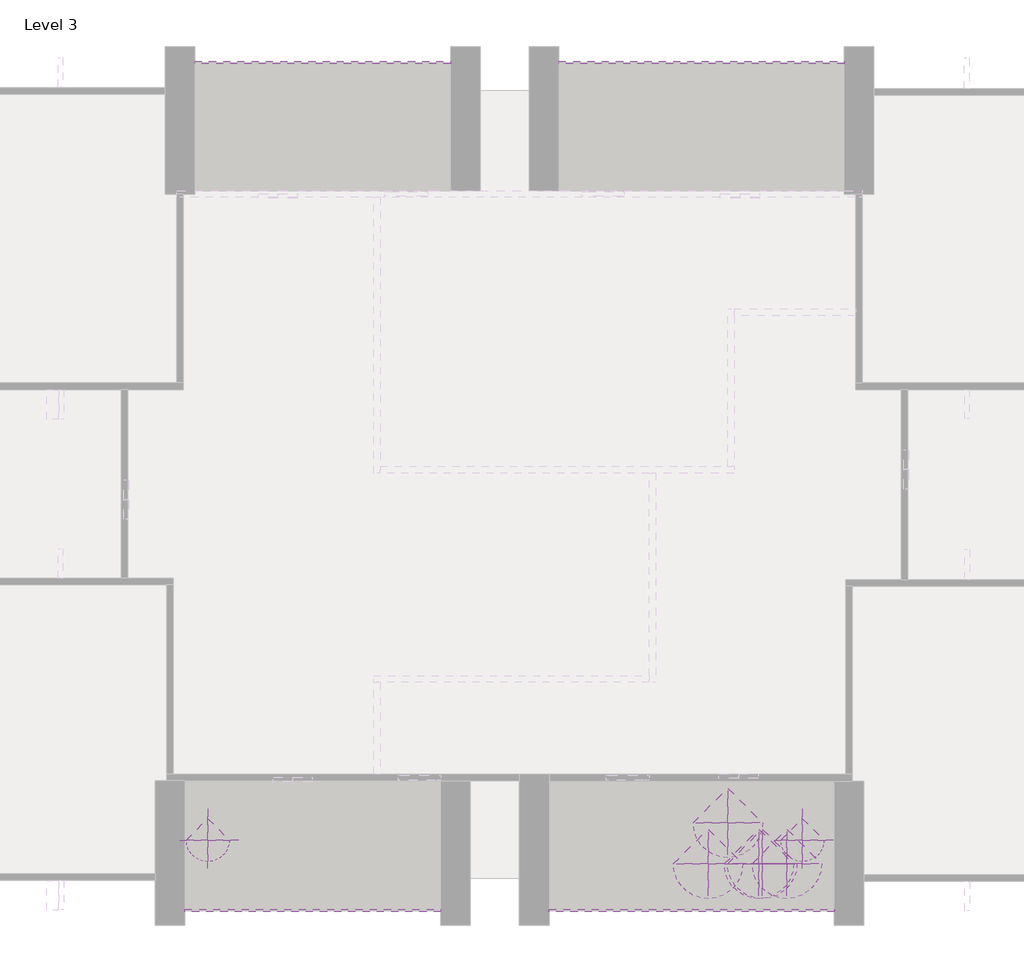
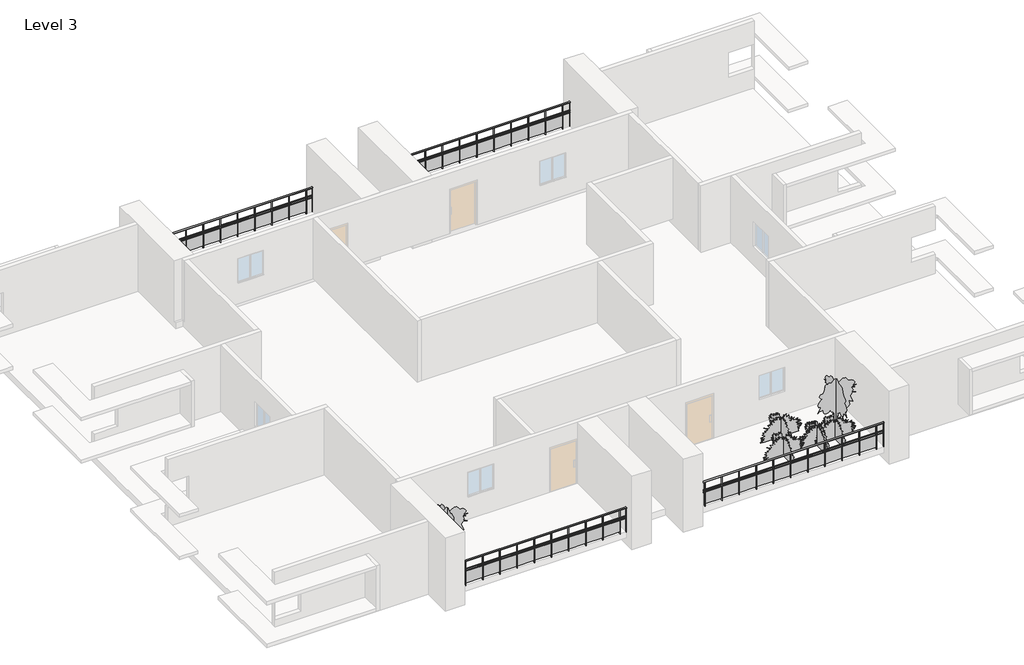
# One storey, part 4 of 4: 7 geographic elements, 4 railings.
"""IFC4 building model written with IfcOpenShell, lengths in millimetres."""

from ifc_helpers import new_model, si_unit, point, frame, origin, place, context, project, spatial, polyline, ellipse_curve, trimmed, outline, extrude, transform, mapped, element, save
from ifc_brep_helpers import plane_surface, extruded_surface, advanced_brep
from components import geographic_element_3d6ded1d, rpc_tree_tropical_d7a905c7

model = new_model("IFC4")

# Units and contexts
model_context = context("Model", 3, world=origin())
ifc_project = project(units=[si_unit("LENGTHUNIT", "METRE", prefix="MILLI")], contexts=[model_context])

# Site, building, storey
site = spatial("IfcSite", under=ifc_project)
building = spatial("IfcBuilding", under=site)
storey = spatial("IfcBuildingStorey", under=building, Name="Level 3", Elevation=6096.0)

# Geographic elements
placement = place(None, origin())
geographic_element_shape = geographic_element_3d6ded1d(model_context)
element("IfcGeographicElement", 1, ObjectType="RPC Shrub : Fountain Grass 3'-6\"", at=placement, inside=storey, context=model_context, shape_type="MappedRepresentation", body=[
    mapped(geographic_element_shape, transform((9500.2520665, -7929.230811, 7315.2), x_axis=(1.0, 0.0, 0.0), y_axis=(0.0, 1.0, 0.0), z_axis=(0.0, 0.0, 1.0))),
])
element("IfcGeographicElement", 2, ObjectType="RPC Shrub : Fountain Grass 3'-6\"", at=placement, inside=storey, context=model_context, shape_type="MappedRepresentation", body=[
    mapped(geographic_element_shape, transform((11938.6520665, -7929.230811, 7315.2), x_axis=(1.0, 0.0, 0.0), y_axis=(0.0, 1.0, 0.0), z_axis=(0.0, 0.0, 1.0))),
])
element("IfcGeographicElement", 3, ObjectType="RPC Shrub : Fountain Grass 3'-6\"", at=placement, inside=storey, context=model_context, shape_type="MappedRepresentation", body=[
    mapped(geographic_element_shape, transform((11176.6520665, -7929.230811, 7315.2), x_axis=(1.0, 0.0, 0.0), y_axis=(0.0, 1.0, 0.0), z_axis=(0.0, 0.0, 1.0))),
])
element("IfcGeographicElement", 4, ObjectType="RPC Shrub : Fountain Grass 3'-6\"", at=placement, inside=storey, context=model_context, shape_type="MappedRepresentation", body=[
    mapped(geographic_element_shape, transform((11075.0520665, -7929.230811, 7315.2), x_axis=(1.0, 0.0, 0.0), y_axis=(0.0, 1.0, 0.0), z_axis=(0.0, 0.0, 1.0))),
])
element("IfcGeographicElement", 5, ObjectType="RPC Shrub : Fountain Grass 3'-6\"", at=placement, inside=storey, context=model_context, shape_type="MappedRepresentation", body=[
    mapped(geographic_element_shape, transform((10109.8520665, -6659.230811, 7315.2), x_axis=(1.0, 0.0, 0.0), y_axis=(0.0, 1.0, 0.0), z_axis=(0.0, 0.0, 1.0))),
])
rpc_tree_tropical_shape = rpc_tree_tropical_d7a905c7(model_context)
element("IfcGeographicElement", 6, ObjectType="RPC Tree - Tropical", at=placement, inside=storey, context=model_context, shape_type="MappedRepresentation", body=[
    mapped(rpc_tree_tropical_shape, transform((-5993.7479335, -7192.630811, 7315.2), x_axis=(1.0, 0.0, 0.0), y_axis=(0.0, 1.0, 0.0), z_axis=(0.0, 0.0, 1.0))),
])
element("IfcGeographicElement", 7, ObjectType="RPC Tree - Tropical", at=placement, inside=storey, context=model_context, shape_type="MappedRepresentation", body=[
    mapped(rpc_tree_tropical_shape, transform((12421.2520665, -7192.630811, 7315.2), x_axis=(1.0, 0.0, 0.0), y_axis=(0.0, 1.0, 0.0), z_axis=(0.0, 0.0, 1.0))),
])

# Railings
element("IfcRailing", 8, ObjectType="Glass Panel - Bottom Fill", at=placement, inside=storey, context=model_context, shape_type="SolidModel", body=[
    advanced_brep(
    [(-6704.9479335, -9342.282663, 8534.4), (-6704.9479335, -9418.482663, 8534.4), (1219.8520665, -9342.282663, 8534.4), (1219.8520665, -9418.482663, 8534.4)],
    [
        (0, 1, ellipse_curve(frame((-6704.9479335, -9380.382663, 8534.4), z_axis=(-1.0, 0.0, 0.0), x_axis=(0.0, -1.0, 0.0)), 38.1, 28.575)),
        (1, 0, ellipse_curve(frame((-6704.9479335, -9380.382663, 8534.4), z_axis=(-1.0, 0.0, 0.0), x_axis=(0.0, -1.0, 0.0)), 38.1, 28.575)),
        (2, 3, ellipse_curve(frame((1219.8520665, -9380.382663, 8534.4), z_axis=(1.0, 0.0, 0.0), x_axis=(0.0, -1.0, 0.0)), 38.1, 28.575)),
        (3, 2, ellipse_curve(frame((1219.8520665, -9380.382663, 8534.4), z_axis=(1.0, 0.0, 0.0), x_axis=(0.0, -1.0, 0.0)), 38.1, 28.575)),
        (0, 2),
        (3, 1),
    ],
    [
        plane_surface(frame((-6704.9479335, -9380.382663, 8534.4), z_axis=(-1.0, 0.0, 0.0), x_axis=(0.0, 1.0, 0.0))),
        plane_surface(frame((1219.8520665, -9380.382663, 8534.4), z_axis=(1.0, 0.0, 0.0), x_axis=(0.0, 1.0, 0.0))),
        extruded_surface(trimmed(ellipse_curve(frame((1219.8520665, -9380.382663, 8534.4), z_axis=(-1.0, 0.0, 0.0), x_axis=(0.0, -1.0, 0.0)), 38.1, 28.575), [point((1219.8520665, -9342.282663, 8534.4))], [point((1219.8520665, -9418.482663, 8534.4))], True, "CARTESIAN"), (-7924.799999999999, 0.0, 0.0), 7924.799999999999),
        extruded_surface(trimmed(ellipse_curve(frame((1219.8520665, -9380.382663, 8534.4), z_axis=(-1.0, 0.0, 0.0), x_axis=(0.0, -1.0, 0.0)), 38.1, 28.575), [point((1219.8520665, -9418.482663, 8534.4))], [point((1219.8520665, -9342.282663, 8534.4))], True, "CARTESIAN"), (-7924.799999999999, 0.0, 0.0), 7924.799999999999),
    ],
    [
        (0, [[1, 2]]),
        (1, [[3, 4]]),
        (2, [[-1, 5, -4, 6]]),
        (3, [[-2, -6, -3, -5]]),
    ],
),
    extrude(outline(polyline([(-6704.9479335, -9393.082663), (-6704.9479335, -9367.682663), (1219.8520665, -9367.682663), (1219.8520665, -9393.082663), (-6704.9479335, -9393.082663)])), frame((0.0, 0.0, 8115.3), z_axis=(0.0, 0.0, 1.0), x_axis=(1.0, 0.0, 0.0)), (0.0, 0.0, 1.0), 25.4),
    extrude(outline(polyline([(-6704.9479335, -9393.082663), (-6704.9479335, -9367.682663), (1219.8520665, -9367.682663), (1219.8520665, -9393.082663), (-6704.9479335, -9393.082663)])), frame((0.0, 0.0, 8013.7), z_axis=(0.0, 0.0, 1.0), x_axis=(1.0, 0.0, 0.0)), (0.0, 0.0, 1.0), 25.4),
    extrude(outline(polyline([(908.7020665, -9405.782663), (908.7020665, -9354.982663), (921.4020665, -9354.982663), (921.4020665, -9405.782663), (908.7020665, -9405.782663)])), frame((0.0, 0.0, 7315.2), z_axis=(0.0, 0.0, 1.0), x_axis=(1.0, 0.0, 0.0)), (0.0, 0.0, 1.0), 1190.4788223),
    extrude(outline(polyline([(102.2520665, -9373.847506), (915.0520665, -9373.847506), (915.0520665, -9380.197506), (102.2520665, -9380.197506), (102.2520665, -9373.847506)])), frame((0.0, 0.0, 7416.8), z_axis=(0.0, 0.0, 1.0), x_axis=(1.0, 0.0, 0.0)), (0.0, 0.0, 1.0), 596.9),
    extrude(outline(polyline([(95.9020665, -9405.782663), (95.9020665, -9354.982663), (108.6020665, -9354.982663), (108.6020665, -9405.782663), (95.9020665, -9405.782663)])), frame((0.0, 0.0, 7315.2), z_axis=(0.0, 0.0, 1.0), x_axis=(1.0, 0.0, 0.0)), (0.0, 0.0, 1.0), 1190.4788223),
    extrude(outline(polyline([(-710.5479335, -9373.847506), (102.2520665, -9373.847506), (102.2520665, -9380.197506), (-710.5479335, -9380.197506), (-710.5479335, -9373.847506)])), frame((0.0, 0.0, 7416.8), z_axis=(0.0, 0.0, 1.0), x_axis=(1.0, 0.0, 0.0)), (0.0, 0.0, 1.0), 596.9),
    extrude(outline(polyline([(-716.8979335, -9405.782663), (-716.8979335, -9354.982663), (-704.1979335, -9354.982663), (-704.1979335, -9405.782663), (-716.8979335, -9405.782663)])), frame((0.0, 0.0, 7315.2), z_axis=(0.0, 0.0, 1.0), x_axis=(1.0, 0.0, 0.0)), (0.0, 0.0, 1.0), 1190.4788223),
    extrude(outline(polyline([(-1523.3479335, -9373.847506), (-710.5479335, -9373.847506), (-710.5479335, -9380.197506), (-1523.3479335, -9380.197506), (-1523.3479335, -9373.847506)])), frame((0.0, 0.0, 7416.8), z_axis=(0.0, 0.0, 1.0), x_axis=(1.0, 0.0, 0.0)), (0.0, 0.0, 1.0), 596.9),
    extrude(outline(polyline([(-1529.6979335, -9405.782663), (-1529.6979335, -9354.982663), (-1516.9979335, -9354.982663), (-1516.9979335, -9405.782663), (-1529.6979335, -9405.782663)])), frame((0.0, 0.0, 7315.2), z_axis=(0.0, 0.0, 1.0), x_axis=(1.0, 0.0, 0.0)), (0.0, 0.0, 1.0), 1190.4788223),
    extrude(outline(polyline([(-2336.1479335, -9373.847506), (-1523.3479335, -9373.847506), (-1523.3479335, -9380.197506), (-2336.1479335, -9380.197506), (-2336.1479335, -9373.847506)])), frame((0.0, 0.0, 7416.8), z_axis=(0.0, 0.0, 1.0), x_axis=(1.0, 0.0, 0.0)), (0.0, 0.0, 1.0), 596.9),
    extrude(outline(polyline([(-2342.4979335, -9405.782663), (-2342.4979335, -9354.982663), (-2329.7979335, -9354.982663), (-2329.7979335, -9405.782663), (-2342.4979335, -9405.782663)])), frame((0.0, 0.0, 7315.2), z_axis=(0.0, 0.0, 1.0), x_axis=(1.0, 0.0, 0.0)), (0.0, 0.0, 1.0), 1190.4788223),
    extrude(outline(polyline([(-3148.9479335, -9373.847506), (-2336.1479335, -9373.847506), (-2336.1479335, -9380.197506), (-3148.9479335, -9380.197506), (-3148.9479335, -9373.847506)])), frame((0.0, 0.0, 7416.8), z_axis=(0.0, 0.0, 1.0), x_axis=(1.0, 0.0, 0.0)), (0.0, 0.0, 1.0), 596.9),
    extrude(outline(polyline([(-3155.2979335, -9405.782663), (-3155.2979335, -9354.982663), (-3142.5979335, -9354.982663), (-3142.5979335, -9405.782663), (-3155.2979335, -9405.782663)])), frame((0.0, 0.0, 7315.2), z_axis=(0.0, 0.0, 1.0), x_axis=(1.0, 0.0, 0.0)), (0.0, 0.0, 1.0), 1190.4788223),
    extrude(outline(polyline([(-3961.7479335, -9373.847506), (-3148.9479335, -9373.847506), (-3148.9479335, -9380.197506), (-3961.7479335, -9380.197506), (-3961.7479335, -9373.847506)])), frame((0.0, 0.0, 7416.8), z_axis=(0.0, 0.0, 1.0), x_axis=(1.0, 0.0, 0.0)), (0.0, 0.0, 1.0), 596.9),
    extrude(outline(polyline([(-3968.0979335, -9405.782663), (-3968.0979335, -9354.982663), (-3955.3979335, -9354.982663), (-3955.3979335, -9405.782663), (-3968.0979335, -9405.782663)])), frame((0.0, 0.0, 7315.2), z_axis=(0.0, 0.0, 1.0), x_axis=(1.0, 0.0, 0.0)), (0.0, 0.0, 1.0), 1190.4788223),
    extrude(outline(polyline([(-4774.5479335, -9373.847506), (-3961.7479335, -9373.847506), (-3961.7479335, -9380.197506), (-4774.5479335, -9380.197506), (-4774.5479335, -9373.847506)])), frame((0.0, 0.0, 7416.8), z_axis=(0.0, 0.0, 1.0), x_axis=(1.0, 0.0, 0.0)), (0.0, 0.0, 1.0), 596.9),
    extrude(outline(polyline([(-4780.8979335, -9405.782663), (-4780.8979335, -9354.982663), (-4768.1979335, -9354.982663), (-4768.1979335, -9405.782663), (-4780.8979335, -9405.782663)])), frame((0.0, 0.0, 7315.2), z_axis=(0.0, 0.0, 1.0), x_axis=(1.0, 0.0, 0.0)), (0.0, 0.0, 1.0), 1190.4788223),
    extrude(outline(polyline([(-5587.3479335, -9373.847506), (-4774.5479335, -9373.847506), (-4774.5479335, -9380.197506), (-5587.3479335, -9380.197506), (-5587.3479335, -9373.847506)])), frame((0.0, 0.0, 7416.8), z_axis=(0.0, 0.0, 1.0), x_axis=(1.0, 0.0, 0.0)), (0.0, 0.0, 1.0), 596.9),
    extrude(outline(polyline([(-5593.6979335, -9405.782663), (-5593.6979335, -9354.982663), (-5580.9979335, -9354.982663), (-5580.9979335, -9405.782663), (-5593.6979335, -9405.782663)])), frame((0.0, 0.0, 7315.2), z_axis=(0.0, 0.0, 1.0), x_axis=(1.0, 0.0, 0.0)), (0.0, 0.0, 1.0), 1190.4788223),
    extrude(outline(polyline([(-6400.1479335, -9373.847506), (-5587.3479335, -9373.847506), (-5587.3479335, -9380.197506), (-6400.1479335, -9380.197506), (-6400.1479335, -9373.847506)])), frame((0.0, 0.0, 7416.8), z_axis=(0.0, 0.0, 1.0), x_axis=(1.0, 0.0, 0.0)), (0.0, 0.0, 1.0), 596.9),
    extrude(outline(polyline([(-6406.4979335, -9405.782663), (-6406.4979335, -9354.982663), (-6393.7979335, -9354.982663), (-6393.7979335, -9405.782663), (-6406.4979335, -9405.782663)])), frame((0.0, 0.0, 7315.2), z_axis=(0.0, 0.0, 1.0), x_axis=(1.0, 0.0, 0.0)), (0.0, 0.0, 1.0), 1190.4788223),
    extrude(outline(polyline([(1207.1520665, -9389.907663), (1207.1520665, -9370.857663), (1226.2020665, -9370.857663), (1226.2020665, -9389.907663), (1207.1520665, -9389.907663)])), frame((0.0, 0.0, 7315.2), z_axis=(0.0, 0.0, 1.0), x_axis=(1.0, 0.0, 0.0)), (0.0, 0.0, 1.0), 1190.4788223),
    extrude(outline(polyline([(-6711.2979335, -9389.907663), (-6711.2979335, -9370.857663), (-6692.2479335, -9370.857663), (-6692.2479335, -9389.907663), (-6711.2979335, -9389.907663)])), frame((0.0, 0.0, 7315.2), z_axis=(0.0, 0.0, 1.0), x_axis=(1.0, 0.0, 0.0)), (0.0, 0.0, 1.0), 1190.4788223),
])
element("IfcRailing", 9, ObjectType="Glass Panel - Bottom Fill", at=placement, inside=storey, context=model_context, shape_type="SolidModel", body=[
    advanced_brep(
    [(4572.6520665, -9342.282663, 8534.4), (4572.6520665, -9418.482663, 8534.4), (13411.8520665, -9342.282663, 8534.4), (13411.8520665, -9418.482663, 8534.4)],
    [
        (0, 1, ellipse_curve(frame((4572.6520665, -9380.382663, 8534.4), z_axis=(-1.0, 0.0, 0.0), x_axis=(0.0, -1.0, 0.0)), 38.1, 28.575)),
        (1, 0, ellipse_curve(frame((4572.6520665, -9380.382663, 8534.4), z_axis=(-1.0, 0.0, 0.0), x_axis=(0.0, -1.0, 0.0)), 38.1, 28.575)),
        (2, 3, ellipse_curve(frame((13411.8520665, -9380.382663, 8534.4), z_axis=(1.0, 0.0, 0.0), x_axis=(0.0, -1.0, 0.0)), 38.1, 28.575)),
        (3, 2, ellipse_curve(frame((13411.8520665, -9380.382663, 8534.4), z_axis=(1.0, 0.0, 0.0), x_axis=(0.0, -1.0, 0.0)), 38.1, 28.575)),
        (0, 2),
        (3, 1),
    ],
    [
        plane_surface(frame((4572.6520665, -9380.382663, 8534.4), z_axis=(-1.0, 0.0, 0.0), x_axis=(0.0, 1.0, 0.0))),
        plane_surface(frame((13411.8520665, -9380.382663, 8534.4), z_axis=(1.0, 0.0, 0.0), x_axis=(0.0, 1.0, 0.0))),
        extruded_surface(trimmed(ellipse_curve(frame((13411.8520665, -9380.382663, 8534.4), z_axis=(-1.0, 0.0, 0.0), x_axis=(0.0, -1.0, 0.0)), 38.1, 28.575), [point((13411.8520665, -9342.282663, 8534.4))], [point((13411.8520665, -9418.482663, 8534.4))], True, "CARTESIAN"), (-8839.2, 0.0, 0.0), 8839.2),
        extruded_surface(trimmed(ellipse_curve(frame((13411.8520665, -9380.382663, 8534.4), z_axis=(-1.0, 0.0, 0.0), x_axis=(0.0, -1.0, 0.0)), 38.1, 28.575), [point((13411.8520665, -9418.482663, 8534.4))], [point((13411.8520665, -9342.282663, 8534.4))], True, "CARTESIAN"), (-8839.2, 0.0, 0.0), 8839.2),
    ],
    [
        (0, [[1, 2]]),
        (1, [[3, 4]]),
        (2, [[-1, 5, -4, 6]]),
        (3, [[-2, -6, -3, -5]]),
    ],
),
    extrude(outline(polyline([(4572.6520665, -9393.082663), (4572.6520665, -9367.682663), (13411.8520665, -9367.682663), (13411.8520665, -9393.082663), (4572.6520665, -9393.082663)])), frame((0.0, 0.0, 8115.3), z_axis=(0.0, 0.0, 1.0), x_axis=(1.0, 0.0, 0.0)), (0.0, 0.0, 1.0), 25.4),
    extrude(outline(polyline([(4572.6520665, -9393.082663), (4572.6520665, -9367.682663), (13411.8520665, -9367.682663), (13411.8520665, -9393.082663), (4572.6520665, -9393.082663)])), frame((0.0, 0.0, 8013.7), z_axis=(0.0, 0.0, 1.0), x_axis=(1.0, 0.0, 0.0)), (0.0, 0.0, 1.0), 25.4),
    extrude(outline(polyline([(13049.9020665, -9405.782663), (13049.9020665, -9354.982663), (13062.6020665, -9354.982663), (13062.6020665, -9405.782663), (13049.9020665, -9405.782663)])), frame((0.0, 0.0, 7315.2), z_axis=(0.0, 0.0, 1.0), x_axis=(1.0, 0.0, 0.0)), (0.0, 0.0, 1.0), 1190.4788223),
    extrude(outline(polyline([(12243.4520665, -9373.847506), (13056.2520665, -9373.847506), (13056.2520665, -9380.197506), (12243.4520665, -9380.197506), (12243.4520665, -9373.847506)])), frame((0.0, 0.0, 7416.8), z_axis=(0.0, 0.0, 1.0), x_axis=(1.0, 0.0, 0.0)), (0.0, 0.0, 1.0), 596.9),
    extrude(outline(polyline([(12237.1020665, -9405.782663), (12237.1020665, -9354.982663), (12249.8020665, -9354.982663), (12249.8020665, -9405.782663), (12237.1020665, -9405.782663)])), frame((0.0, 0.0, 7315.2), z_axis=(0.0, 0.0, 1.0), x_axis=(1.0, 0.0, 0.0)), (0.0, 0.0, 1.0), 1190.4788223),
    extrude(outline(polyline([(11430.6520665, -9373.847506), (12243.4520665, -9373.847506), (12243.4520665, -9380.197506), (11430.6520665, -9380.197506), (11430.6520665, -9373.847506)])), frame((0.0, 0.0, 7416.8), z_axis=(0.0, 0.0, 1.0), x_axis=(1.0, 0.0, 0.0)), (0.0, 0.0, 1.0), 596.9),
    extrude(outline(polyline([(11424.3020665, -9405.782663), (11424.3020665, -9354.982663), (11437.0020665, -9354.982663), (11437.0020665, -9405.782663), (11424.3020665, -9405.782663)])), frame((0.0, 0.0, 7315.2), z_axis=(0.0, 0.0, 1.0), x_axis=(1.0, 0.0, 0.0)), (0.0, 0.0, 1.0), 1190.4788223),
    extrude(outline(polyline([(10617.8520665, -9373.847506), (11430.6520665, -9373.847506), (11430.6520665, -9380.197506), (10617.8520665, -9380.197506), (10617.8520665, -9373.847506)])), frame((0.0, 0.0, 7416.8), z_axis=(0.0, 0.0, 1.0), x_axis=(1.0, 0.0, 0.0)), (0.0, 0.0, 1.0), 596.9),
    extrude(outline(polyline([(10611.5020665, -9405.782663), (10611.5020665, -9354.982663), (10624.2020665, -9354.982663), (10624.2020665, -9405.782663), (10611.5020665, -9405.782663)])), frame((0.0, 0.0, 7315.2), z_axis=(0.0, 0.0, 1.0), x_axis=(1.0, 0.0, 0.0)), (0.0, 0.0, 1.0), 1190.4788223),
    extrude(outline(polyline([(9805.0520665, -9373.847506), (10617.8520665, -9373.847506), (10617.8520665, -9380.197506), (9805.0520665, -9380.197506), (9805.0520665, -9373.847506)])), frame((0.0, 0.0, 7416.8), z_axis=(0.0, 0.0, 1.0), x_axis=(1.0, 0.0, 0.0)), (0.0, 0.0, 1.0), 596.9),
    extrude(outline(polyline([(9798.7020665, -9405.782663), (9798.7020665, -9354.982663), (9811.4020665, -9354.982663), (9811.4020665, -9405.782663), (9798.7020665, -9405.782663)])), frame((0.0, 0.0, 7315.2), z_axis=(0.0, 0.0, 1.0), x_axis=(1.0, 0.0, 0.0)), (0.0, 0.0, 1.0), 1190.4788223),
    extrude(outline(polyline([(8992.2520665, -9373.847506), (9805.0520665, -9373.847506), (9805.0520665, -9380.197506), (8992.2520665, -9380.197506), (8992.2520665, -9373.847506)])), frame((0.0, 0.0, 7416.8), z_axis=(0.0, 0.0, 1.0), x_axis=(1.0, 0.0, 0.0)), (0.0, 0.0, 1.0), 596.9),
    extrude(outline(polyline([(8985.9020665, -9405.782663), (8985.9020665, -9354.982663), (8998.6020665, -9354.982663), (8998.6020665, -9405.782663), (8985.9020665, -9405.782663)])), frame((0.0, 0.0, 7315.2), z_axis=(0.0, 0.0, 1.0), x_axis=(1.0, 0.0, 0.0)), (0.0, 0.0, 1.0), 1190.4788223),
    extrude(outline(polyline([(8179.4520665, -9373.847506), (8992.2520665, -9373.847506), (8992.2520665, -9380.197506), (8179.4520665, -9380.197506), (8179.4520665, -9373.847506)])), frame((0.0, 0.0, 7416.8), z_axis=(0.0, 0.0, 1.0), x_axis=(1.0, 0.0, 0.0)), (0.0, 0.0, 1.0), 596.9),
    extrude(outline(polyline([(8173.1020665, -9405.782663), (8173.1020665, -9354.982663), (8185.8020665, -9354.982663), (8185.8020665, -9405.782663), (8173.1020665, -9405.782663)])), frame((0.0, 0.0, 7315.2), z_axis=(0.0, 0.0, 1.0), x_axis=(1.0, 0.0, 0.0)), (0.0, 0.0, 1.0), 1190.4788223),
    extrude(outline(polyline([(7366.6520665, -9373.847506), (8179.4520665, -9373.847506), (8179.4520665, -9380.197506), (7366.6520665, -9380.197506), (7366.6520665, -9373.847506)])), frame((0.0, 0.0, 7416.8), z_axis=(0.0, 0.0, 1.0), x_axis=(1.0, 0.0, 0.0)), (0.0, 0.0, 1.0), 596.9),
    extrude(outline(polyline([(7360.3020665, -9405.782663), (7360.3020665, -9354.982663), (7373.0020665, -9354.982663), (7373.0020665, -9405.782663), (7360.3020665, -9405.782663)])), frame((0.0, 0.0, 7315.2), z_axis=(0.0, 0.0, 1.0), x_axis=(1.0, 0.0, 0.0)), (0.0, 0.0, 1.0), 1190.4788223),
    extrude(outline(polyline([(6553.8520665, -9373.847506), (7366.6520665, -9373.847506), (7366.6520665, -9380.197506), (6553.8520665, -9380.197506), (6553.8520665, -9373.847506)])), frame((0.0, 0.0, 7416.8), z_axis=(0.0, 0.0, 1.0), x_axis=(1.0, 0.0, 0.0)), (0.0, 0.0, 1.0), 596.9),
    extrude(outline(polyline([(6547.5020665, -9405.782663), (6547.5020665, -9354.982663), (6560.2020665, -9354.982663), (6560.2020665, -9405.782663), (6547.5020665, -9405.782663)])), frame((0.0, 0.0, 7315.2), z_axis=(0.0, 0.0, 1.0), x_axis=(1.0, 0.0, 0.0)), (0.0, 0.0, 1.0), 1190.4788223),
    extrude(outline(polyline([(5741.0520665, -9373.847506), (6553.8520665, -9373.847506), (6553.8520665, -9380.197506), (5741.0520665, -9380.197506), (5741.0520665, -9373.847506)])), frame((0.0, 0.0, 7416.8), z_axis=(0.0, 0.0, 1.0), x_axis=(1.0, 0.0, 0.0)), (0.0, 0.0, 1.0), 596.9),
    extrude(outline(polyline([(5734.7020665, -9405.782663), (5734.7020665, -9354.982663), (5747.4020665, -9354.982663), (5747.4020665, -9405.782663), (5734.7020665, -9405.782663)])), frame((0.0, 0.0, 7315.2), z_axis=(0.0, 0.0, 1.0), x_axis=(1.0, 0.0, 0.0)), (0.0, 0.0, 1.0), 1190.4788223),
    extrude(outline(polyline([(4928.2520665, -9373.847506), (5741.0520665, -9373.847506), (5741.0520665, -9380.197506), (4928.2520665, -9380.197506), (4928.2520665, -9373.847506)])), frame((0.0, 0.0, 7416.8), z_axis=(0.0, 0.0, 1.0), x_axis=(1.0, 0.0, 0.0)), (0.0, 0.0, 1.0), 596.9),
    extrude(outline(polyline([(4921.9020665, -9405.782663), (4921.9020665, -9354.982663), (4934.6020665, -9354.982663), (4934.6020665, -9405.782663), (4921.9020665, -9405.782663)])), frame((0.0, 0.0, 7315.2), z_axis=(0.0, 0.0, 1.0), x_axis=(1.0, 0.0, 0.0)), (0.0, 0.0, 1.0), 1190.4788223),
    extrude(outline(polyline([(13399.1520665, -9389.907663), (13399.1520665, -9370.857663), (13418.2020665, -9370.857663), (13418.2020665, -9389.907663), (13399.1520665, -9389.907663)])), frame((0.0, 0.0, 7315.2), z_axis=(0.0, 0.0, 1.0), x_axis=(1.0, 0.0, 0.0)), (0.0, 0.0, 1.0), 1190.4788223),
    extrude(outline(polyline([(4566.3020665, -9389.907663), (4566.3020665, -9370.857663), (4585.3520665, -9370.857663), (4585.3520665, -9389.907663), (4566.3020665, -9389.907663)])), frame((0.0, 0.0, 7315.2), z_axis=(0.0, 0.0, 1.0), x_axis=(1.0, 0.0, 0.0)), (0.0, 0.0, 1.0), 1190.4788223),
])
element("IfcRailing", 10, ObjectType="Glass Panel - Bottom Fill", at=placement, inside=storey, context=model_context, shape_type="SolidModel", body=[
    advanced_brep(
    [(-6400.1479335, 16924.2559451, 8534.4), (-6400.1479335, 16848.0559451, 8534.4), (1524.6520665, 16924.2559451, 8534.4), (1524.6520665, 16848.0559451, 8534.4)],
    [
        (0, 1, ellipse_curve(frame((-6400.1479335, 16886.1559451, 8534.4), z_axis=(-1.0, 0.0, 0.0), x_axis=(0.0, -1.0, 0.0)), 38.1, 28.575)),
        (1, 0, ellipse_curve(frame((-6400.1479335, 16886.1559451, 8534.4), z_axis=(-1.0, 0.0, 0.0), x_axis=(0.0, -1.0, 0.0)), 38.1, 28.575)),
        (2, 3, ellipse_curve(frame((1524.6520665, 16886.1559451, 8534.4), z_axis=(1.0, 0.0, 0.0), x_axis=(0.0, -1.0, 0.0)), 38.1, 28.575)),
        (3, 2, ellipse_curve(frame((1524.6520665, 16886.1559451, 8534.4), z_axis=(1.0, 0.0, 0.0), x_axis=(0.0, -1.0, 0.0)), 38.1, 28.575)),
        (0, 2),
        (3, 1),
    ],
    [
        plane_surface(frame((-6400.1479335, 16886.1559451, 8534.4), z_axis=(-1.0, 0.0, 0.0), x_axis=(0.0, 1.0, 0.0))),
        plane_surface(frame((1524.6520665, 16886.1559451, 8534.4), z_axis=(1.0, 0.0, 0.0), x_axis=(0.0, 1.0, 0.0))),
        extruded_surface(trimmed(ellipse_curve(frame((1524.6520665, 16886.1559451, 8534.4), z_axis=(-1.0, 0.0, 0.0), x_axis=(0.0, -1.0, 0.0)), 38.1, 28.575), [point((1524.6520665, 16924.2559451, 8534.4))], [point((1524.6520665, 16848.0559451, 8534.4))], True, "CARTESIAN"), (-7924.8, 0.0, 0.0), 7924.8),
        extruded_surface(trimmed(ellipse_curve(frame((1524.6520665, 16886.1559451, 8534.4), z_axis=(-1.0, 0.0, 0.0), x_axis=(0.0, -1.0, 0.0)), 38.1, 28.575), [point((1524.6520665, 16848.0559451, 8534.4))], [point((1524.6520665, 16924.2559451, 8534.4))], True, "CARTESIAN"), (-7924.8, 0.0, 0.0), 7924.8),
    ],
    [
        (0, [[1, 2]]),
        (1, [[3, 4]]),
        (2, [[-1, 5, -4, 6]]),
        (3, [[-2, -6, -3, -5]]),
    ],
),
    extrude(outline(polyline([(-6400.1479335, 16873.4559451), (-6400.1479335, 16898.8559451), (1524.6520665, 16898.8559451), (1524.6520665, 16873.4559451), (-6400.1479335, 16873.4559451)])), frame((0.0, 0.0, 8115.3), z_axis=(0.0, 0.0, 1.0), x_axis=(1.0, 0.0, 0.0)), (0.0, 0.0, 1.0), 25.4),
    extrude(outline(polyline([(-6400.1479335, 16873.4559451), (-6400.1479335, 16898.8559451), (1524.6520665, 16898.8559451), (1524.6520665, 16873.4559451), (-6400.1479335, 16873.4559451)])), frame((0.0, 0.0, 8013.7), z_axis=(0.0, 0.0, 1.0), x_axis=(1.0, 0.0, 0.0)), (0.0, 0.0, 1.0), 25.4),
    extrude(outline(polyline([(1213.5020665, 16860.7559451), (1213.5020665, 16911.5559451), (1226.2020665, 16911.5559451), (1226.2020665, 16860.7559451), (1213.5020665, 16860.7559451)])), frame((0.0, 0.0, 7315.2), z_axis=(0.0, 0.0, 1.0), x_axis=(1.0, 0.0, 0.0)), (0.0, 0.0, 1.0), 1190.4788223),
    extrude(outline(polyline([(407.0520665, 16892.6911021), (1219.8520665, 16892.6911021), (1219.8520665, 16886.3411021), (407.0520665, 16886.3411021), (407.0520665, 16892.6911021)])), frame((0.0, 0.0, 7416.8), z_axis=(0.0, 0.0, 1.0), x_axis=(1.0, 0.0, 0.0)), (0.0, 0.0, 1.0), 596.9),
    extrude(outline(polyline([(400.7020665, 16860.7559451), (400.7020665, 16911.5559451), (413.4020665, 16911.5559451), (413.4020665, 16860.7559451), (400.7020665, 16860.7559451)])), frame((0.0, 0.0, 7315.2), z_axis=(0.0, 0.0, 1.0), x_axis=(1.0, 0.0, 0.0)), (0.0, 0.0, 1.0), 1190.4788223),
    extrude(outline(polyline([(-405.7479335, 16892.6911021), (407.0520665, 16892.6911021), (407.0520665, 16886.3411021), (-405.7479335, 16886.3411021), (-405.7479335, 16892.6911021)])), frame((0.0, 0.0, 7416.8), z_axis=(0.0, 0.0, 1.0), x_axis=(1.0, 0.0, 0.0)), (0.0, 0.0, 1.0), 596.9),
    extrude(outline(polyline([(-412.0979335, 16860.7559451), (-412.0979335, 16911.5559451), (-399.3979335, 16911.5559451), (-399.3979335, 16860.7559451), (-412.0979335, 16860.7559451)])), frame((0.0, 0.0, 7315.2), z_axis=(0.0, 0.0, 1.0), x_axis=(1.0, 0.0, 0.0)), (0.0, 0.0, 1.0), 1190.4788223),
    extrude(outline(polyline([(-1218.5479335, 16892.6911021), (-405.7479335, 16892.6911021), (-405.7479335, 16886.3411021), (-1218.5479335, 16886.3411021), (-1218.5479335, 16892.6911021)])), frame((0.0, 0.0, 7416.8), z_axis=(0.0, 0.0, 1.0), x_axis=(1.0, 0.0, 0.0)), (0.0, 0.0, 1.0), 596.9),
    extrude(outline(polyline([(-1224.8979335, 16860.7559451), (-1224.8979335, 16911.5559451), (-1212.1979335, 16911.5559451), (-1212.1979335, 16860.7559451), (-1224.8979335, 16860.7559451)])), frame((0.0, 0.0, 7315.2), z_axis=(0.0, 0.0, 1.0), x_axis=(1.0, 0.0, 0.0)), (0.0, 0.0, 1.0), 1190.4788223),
    extrude(outline(polyline([(-2031.3479335, 16892.6911021), (-1218.5479335, 16892.6911021), (-1218.5479335, 16886.3411021), (-2031.3479335, 16886.3411021), (-2031.3479335, 16892.6911021)])), frame((0.0, 0.0, 7416.8), z_axis=(0.0, 0.0, 1.0), x_axis=(1.0, 0.0, 0.0)), (0.0, 0.0, 1.0), 596.9),
    extrude(outline(polyline([(-2037.6979335, 16860.7559451), (-2037.6979335, 16911.5559451), (-2024.9979335, 16911.5559451), (-2024.9979335, 16860.7559451), (-2037.6979335, 16860.7559451)])), frame((0.0, 0.0, 7315.2), z_axis=(0.0, 0.0, 1.0), x_axis=(1.0, 0.0, 0.0)), (0.0, 0.0, 1.0), 1190.4788223),
    extrude(outline(polyline([(-2844.1479335, 16892.6911021), (-2031.3479335, 16892.6911021), (-2031.3479335, 16886.3411021), (-2844.1479335, 16886.3411021), (-2844.1479335, 16892.6911021)])), frame((0.0, 0.0, 7416.8), z_axis=(0.0, 0.0, 1.0), x_axis=(1.0, 0.0, 0.0)), (0.0, 0.0, 1.0), 596.9),
    extrude(outline(polyline([(-2850.4979335, 16860.7559451), (-2850.4979335, 16911.5559451), (-2837.7979335, 16911.5559451), (-2837.7979335, 16860.7559451), (-2850.4979335, 16860.7559451)])), frame((0.0, 0.0, 7315.2), z_axis=(0.0, 0.0, 1.0), x_axis=(1.0, 0.0, 0.0)), (0.0, 0.0, 1.0), 1190.4788223),
    extrude(outline(polyline([(-3656.9479335, 16892.6911021), (-2844.1479335, 16892.6911021), (-2844.1479335, 16886.3411021), (-3656.9479335, 16886.3411021), (-3656.9479335, 16892.6911021)])), frame((0.0, 0.0, 7416.8), z_axis=(0.0, 0.0, 1.0), x_axis=(1.0, 0.0, 0.0)), (0.0, 0.0, 1.0), 596.9),
    extrude(outline(polyline([(-3663.2979335, 16860.7559451), (-3663.2979335, 16911.5559451), (-3650.5979335, 16911.5559451), (-3650.5979335, 16860.7559451), (-3663.2979335, 16860.7559451)])), frame((0.0, 0.0, 7315.2), z_axis=(0.0, 0.0, 1.0), x_axis=(1.0, 0.0, 0.0)), (0.0, 0.0, 1.0), 1190.4788223),
    extrude(outline(polyline([(-4469.7479335, 16892.6911021), (-3656.9479335, 16892.6911021), (-3656.9479335, 16886.3411021), (-4469.7479335, 16886.3411021), (-4469.7479335, 16892.6911021)])), frame((0.0, 0.0, 7416.8), z_axis=(0.0, 0.0, 1.0), x_axis=(1.0, 0.0, 0.0)), (0.0, 0.0, 1.0), 596.9),
    extrude(outline(polyline([(-4476.0979335, 16860.7559451), (-4476.0979335, 16911.5559451), (-4463.3979335, 16911.5559451), (-4463.3979335, 16860.7559451), (-4476.0979335, 16860.7559451)])), frame((0.0, 0.0, 7315.2), z_axis=(0.0, 0.0, 1.0), x_axis=(1.0, 0.0, 0.0)), (0.0, 0.0, 1.0), 1190.4788223),
    extrude(outline(polyline([(-5282.5479335, 16892.6911021), (-4469.7479335, 16892.6911021), (-4469.7479335, 16886.3411021), (-5282.5479335, 16886.3411021), (-5282.5479335, 16892.6911021)])), frame((0.0, 0.0, 7416.8), z_axis=(0.0, 0.0, 1.0), x_axis=(1.0, 0.0, 0.0)), (0.0, 0.0, 1.0), 596.9),
    extrude(outline(polyline([(-5288.8979335, 16860.7559451), (-5288.8979335, 16911.5559451), (-5276.1979335, 16911.5559451), (-5276.1979335, 16860.7559451), (-5288.8979335, 16860.7559451)])), frame((0.0, 0.0, 7315.2), z_axis=(0.0, 0.0, 1.0), x_axis=(1.0, 0.0, 0.0)), (0.0, 0.0, 1.0), 1190.4788223),
    extrude(outline(polyline([(-6095.3479335, 16892.6911021), (-5282.5479335, 16892.6911021), (-5282.5479335, 16886.3411021), (-6095.3479335, 16886.3411021), (-6095.3479335, 16892.6911021)])), frame((0.0, 0.0, 7416.8), z_axis=(0.0, 0.0, 1.0), x_axis=(1.0, 0.0, 0.0)), (0.0, 0.0, 1.0), 596.9),
    extrude(outline(polyline([(-6101.6979335, 16860.7559451), (-6101.6979335, 16911.5559451), (-6088.9979335, 16911.5559451), (-6088.9979335, 16860.7559451), (-6101.6979335, 16860.7559451)])), frame((0.0, 0.0, 7315.2), z_axis=(0.0, 0.0, 1.0), x_axis=(1.0, 0.0, 0.0)), (0.0, 0.0, 1.0), 1190.4788223),
    extrude(outline(polyline([(1511.9520665, 16876.6309451), (1511.9520665, 16895.6809451), (1531.0020665, 16895.6809451), (1531.0020665, 16876.6309451), (1511.9520665, 16876.6309451)])), frame((0.0, 0.0, 7315.2), z_axis=(0.0, 0.0, 1.0), x_axis=(1.0, 0.0, 0.0)), (0.0, 0.0, 1.0), 1190.4788223),
    extrude(outline(polyline([(-6406.4979335, 16876.6309451), (-6406.4979335, 16895.6809451), (-6387.4479335, 16895.6809451), (-6387.4479335, 16876.6309451), (-6406.4979335, 16876.6309451)])), frame((0.0, 0.0, 7315.2), z_axis=(0.0, 0.0, 1.0), x_axis=(1.0, 0.0, 0.0)), (0.0, 0.0, 1.0), 1190.4788223),
])
element("IfcRailing", 11, ObjectType="Glass Panel - Bottom Fill", at=placement, inside=storey, context=model_context, shape_type="SolidModel", body=[
    advanced_brep(
    [(4877.4520665, 16924.2559451, 8534.4), (4877.4520665, 16848.0559451, 8534.4), (13716.6520665, 16924.2559451, 8534.4), (13716.6520665, 16848.0559451, 8534.4)],
    [
        (0, 1, ellipse_curve(frame((4877.4520665, 16886.1559451, 8534.4), z_axis=(-1.0, 0.0, 0.0), x_axis=(0.0, -1.0, 0.0)), 38.1, 28.575)),
        (1, 0, ellipse_curve(frame((4877.4520665, 16886.1559451, 8534.4), z_axis=(-1.0, 0.0, 0.0), x_axis=(0.0, -1.0, 0.0)), 38.1, 28.575)),
        (2, 3, ellipse_curve(frame((13716.6520665, 16886.1559451, 8534.4), z_axis=(1.0, 0.0, 0.0), x_axis=(0.0, -1.0, 0.0)), 38.1, 28.575)),
        (3, 2, ellipse_curve(frame((13716.6520665, 16886.1559451, 8534.4), z_axis=(1.0, 0.0, 0.0), x_axis=(0.0, -1.0, 0.0)), 38.1, 28.575)),
        (0, 2),
        (3, 1),
    ],
    [
        plane_surface(frame((4877.4520665, 16886.1559451, 8534.4), z_axis=(-1.0, 0.0, 0.0), x_axis=(0.0, 1.0, 0.0))),
        plane_surface(frame((13716.6520665, 16886.1559451, 8534.4), z_axis=(1.0, 0.0, 0.0), x_axis=(0.0, 1.0, 0.0))),
        extruded_surface(trimmed(ellipse_curve(frame((13716.6520665, 16886.1559451, 8534.4), z_axis=(-1.0, 0.0, 0.0), x_axis=(0.0, -1.0, 0.0)), 38.1, 28.575), [point((13716.6520665, 16924.2559451, 8534.4))], [point((13716.6520665, 16848.0559451, 8534.4))], True, "CARTESIAN"), (-8839.2, 0.0, 0.0), 8839.2),
        extruded_surface(trimmed(ellipse_curve(frame((13716.6520665, 16886.1559451, 8534.4), z_axis=(-1.0, 0.0, 0.0), x_axis=(0.0, -1.0, 0.0)), 38.1, 28.575), [point((13716.6520665, 16848.0559451, 8534.4))], [point((13716.6520665, 16924.2559451, 8534.4))], True, "CARTESIAN"), (-8839.2, 0.0, 0.0), 8839.2),
    ],
    [
        (0, [[1, 2]]),
        (1, [[3, 4]]),
        (2, [[-1, 5, -4, 6]]),
        (3, [[-2, -6, -3, -5]]),
    ],
),
    extrude(outline(polyline([(4877.4520665, 16873.4559451), (4877.4520665, 16898.8559451), (13716.6520665, 16898.8559451), (13716.6520665, 16873.4559451), (4877.4520665, 16873.4559451)])), frame((0.0, 0.0, 8115.3), z_axis=(0.0, 0.0, 1.0), x_axis=(1.0, 0.0, 0.0)), (0.0, 0.0, 1.0), 25.4),
    extrude(outline(polyline([(4877.4520665, 16873.4559451), (4877.4520665, 16898.8559451), (13716.6520665, 16898.8559451), (13716.6520665, 16873.4559451), (4877.4520665, 16873.4559451)])), frame((0.0, 0.0, 8013.7), z_axis=(0.0, 0.0, 1.0), x_axis=(1.0, 0.0, 0.0)), (0.0, 0.0, 1.0), 25.4),
    extrude(outline(polyline([(13354.7020665, 16860.7559451), (13354.7020665, 16911.5559451), (13367.4020665, 16911.5559451), (13367.4020665, 16860.7559451), (13354.7020665, 16860.7559451)])), frame((0.0, 0.0, 7315.2), z_axis=(0.0, 0.0, 1.0), x_axis=(1.0, 0.0, 0.0)), (0.0, 0.0, 1.0), 1190.4788223),
    extrude(outline(polyline([(12548.2520665, 16892.6911021), (13361.0520665, 16892.6911021), (13361.0520665, 16886.3411021), (12548.2520665, 16886.3411021), (12548.2520665, 16892.6911021)])), frame((0.0, 0.0, 7416.8), z_axis=(0.0, 0.0, 1.0), x_axis=(1.0, 0.0, 0.0)), (0.0, 0.0, 1.0), 596.9),
    extrude(outline(polyline([(12541.9020665, 16860.7559451), (12541.9020665, 16911.5559451), (12554.6020665, 16911.5559451), (12554.6020665, 16860.7559451), (12541.9020665, 16860.7559451)])), frame((0.0, 0.0, 7315.2), z_axis=(0.0, 0.0, 1.0), x_axis=(1.0, 0.0, 0.0)), (0.0, 0.0, 1.0), 1190.4788223),
    extrude(outline(polyline([(11735.4520665, 16892.6911021), (12548.2520665, 16892.6911021), (12548.2520665, 16886.3411021), (11735.4520665, 16886.3411021), (11735.4520665, 16892.6911021)])), frame((0.0, 0.0, 7416.8), z_axis=(0.0, 0.0, 1.0), x_axis=(1.0, 0.0, 0.0)), (0.0, 0.0, 1.0), 596.9),
    extrude(outline(polyline([(11729.1020665, 16860.7559451), (11729.1020665, 16911.5559451), (11741.8020665, 16911.5559451), (11741.8020665, 16860.7559451), (11729.1020665, 16860.7559451)])), frame((0.0, 0.0, 7315.2), z_axis=(0.0, 0.0, 1.0), x_axis=(1.0, 0.0, 0.0)), (0.0, 0.0, 1.0), 1190.4788223),
    extrude(outline(polyline([(10922.6520665, 16892.6911021), (11735.4520665, 16892.6911021), (11735.4520665, 16886.3411021), (10922.6520665, 16886.3411021), (10922.6520665, 16892.6911021)])), frame((0.0, 0.0, 7416.8), z_axis=(0.0, 0.0, 1.0), x_axis=(1.0, 0.0, 0.0)), (0.0, 0.0, 1.0), 596.9),
    extrude(outline(polyline([(10916.3020665, 16860.7559451), (10916.3020665, 16911.5559451), (10929.0020665, 16911.5559451), (10929.0020665, 16860.7559451), (10916.3020665, 16860.7559451)])), frame((0.0, 0.0, 7315.2), z_axis=(0.0, 0.0, 1.0), x_axis=(1.0, 0.0, 0.0)), (0.0, 0.0, 1.0), 1190.4788223),
    extrude(outline(polyline([(10109.8520665, 16892.6911021), (10922.6520665, 16892.6911021), (10922.6520665, 16886.3411021), (10109.8520665, 16886.3411021), (10109.8520665, 16892.6911021)])), frame((0.0, 0.0, 7416.8), z_axis=(0.0, 0.0, 1.0), x_axis=(1.0, 0.0, 0.0)), (0.0, 0.0, 1.0), 596.9),
    extrude(outline(polyline([(10103.5020665, 16860.7559451), (10103.5020665, 16911.5559451), (10116.2020665, 16911.5559451), (10116.2020665, 16860.7559451), (10103.5020665, 16860.7559451)])), frame((0.0, 0.0, 7315.2), z_axis=(0.0, 0.0, 1.0), x_axis=(1.0, 0.0, 0.0)), (0.0, 0.0, 1.0), 1190.4788223),
    extrude(outline(polyline([(9297.0520665, 16892.6911021), (10109.8520665, 16892.6911021), (10109.8520665, 16886.3411021), (9297.0520665, 16886.3411021), (9297.0520665, 16892.6911021)])), frame((0.0, 0.0, 7416.8), z_axis=(0.0, 0.0, 1.0), x_axis=(1.0, 0.0, 0.0)), (0.0, 0.0, 1.0), 596.9),
    extrude(outline(polyline([(9290.7020665, 16860.7559451), (9290.7020665, 16911.5559451), (9303.4020665, 16911.5559451), (9303.4020665, 16860.7559451), (9290.7020665, 16860.7559451)])), frame((0.0, 0.0, 7315.2), z_axis=(0.0, 0.0, 1.0), x_axis=(1.0, 0.0, 0.0)), (0.0, 0.0, 1.0), 1190.4788223),
    extrude(outline(polyline([(8484.2520665, 16892.6911021), (9297.0520665, 16892.6911021), (9297.0520665, 16886.3411021), (8484.2520665, 16886.3411021), (8484.2520665, 16892.6911021)])), frame((0.0, 0.0, 7416.8), z_axis=(0.0, 0.0, 1.0), x_axis=(1.0, 0.0, 0.0)), (0.0, 0.0, 1.0), 596.9),
    extrude(outline(polyline([(8477.9020665, 16860.7559451), (8477.9020665, 16911.5559451), (8490.6020665, 16911.5559451), (8490.6020665, 16860.7559451), (8477.9020665, 16860.7559451)])), frame((0.0, 0.0, 7315.2), z_axis=(0.0, 0.0, 1.0), x_axis=(1.0, 0.0, 0.0)), (0.0, 0.0, 1.0), 1190.4788223),
    extrude(outline(polyline([(7671.4520665, 16892.6911021), (8484.2520665, 16892.6911021), (8484.2520665, 16886.3411021), (7671.4520665, 16886.3411021), (7671.4520665, 16892.6911021)])), frame((0.0, 0.0, 7416.8), z_axis=(0.0, 0.0, 1.0), x_axis=(1.0, 0.0, 0.0)), (0.0, 0.0, 1.0), 596.9),
    extrude(outline(polyline([(7665.1020665, 16860.7559451), (7665.1020665, 16911.5559451), (7677.8020665, 16911.5559451), (7677.8020665, 16860.7559451), (7665.1020665, 16860.7559451)])), frame((0.0, 0.0, 7315.2), z_axis=(0.0, 0.0, 1.0), x_axis=(1.0, 0.0, 0.0)), (0.0, 0.0, 1.0), 1190.4788223),
    extrude(outline(polyline([(6858.6520665, 16892.6911021), (7671.4520665, 16892.6911021), (7671.4520665, 16886.3411021), (6858.6520665, 16886.3411021), (6858.6520665, 16892.6911021)])), frame((0.0, 0.0, 7416.8), z_axis=(0.0, 0.0, 1.0), x_axis=(1.0, 0.0, 0.0)), (0.0, 0.0, 1.0), 596.9),
    extrude(outline(polyline([(6852.3020665, 16860.7559451), (6852.3020665, 16911.5559451), (6865.0020665, 16911.5559451), (6865.0020665, 16860.7559451), (6852.3020665, 16860.7559451)])), frame((0.0, 0.0, 7315.2), z_axis=(0.0, 0.0, 1.0), x_axis=(1.0, 0.0, 0.0)), (0.0, 0.0, 1.0), 1190.4788223),
    extrude(outline(polyline([(6045.8520665, 16892.6911021), (6858.6520665, 16892.6911021), (6858.6520665, 16886.3411021), (6045.8520665, 16886.3411021), (6045.8520665, 16892.6911021)])), frame((0.0, 0.0, 7416.8), z_axis=(0.0, 0.0, 1.0), x_axis=(1.0, 0.0, 0.0)), (0.0, 0.0, 1.0), 596.9),
    extrude(outline(polyline([(6039.5020665, 16860.7559451), (6039.5020665, 16911.5559451), (6052.2020665, 16911.5559451), (6052.2020665, 16860.7559451), (6039.5020665, 16860.7559451)])), frame((0.0, 0.0, 7315.2), z_axis=(0.0, 0.0, 1.0), x_axis=(1.0, 0.0, 0.0)), (0.0, 0.0, 1.0), 1190.4788223),
    extrude(outline(polyline([(5233.0520665, 16892.6911021), (6045.8520665, 16892.6911021), (6045.8520665, 16886.3411021), (5233.0520665, 16886.3411021), (5233.0520665, 16892.6911021)])), frame((0.0, 0.0, 7416.8), z_axis=(0.0, 0.0, 1.0), x_axis=(1.0, 0.0, 0.0)), (0.0, 0.0, 1.0), 596.9),
    extrude(outline(polyline([(5226.7020665, 16860.7559451), (5226.7020665, 16911.5559451), (5239.4020665, 16911.5559451), (5239.4020665, 16860.7559451), (5226.7020665, 16860.7559451)])), frame((0.0, 0.0, 7315.2), z_axis=(0.0, 0.0, 1.0), x_axis=(1.0, 0.0, 0.0)), (0.0, 0.0, 1.0), 1190.4788223),
    extrude(outline(polyline([(13703.9520665, 16876.6309451), (13703.9520665, 16895.6809451), (13723.0020665, 16895.6809451), (13723.0020665, 16876.6309451), (13703.9520665, 16876.6309451)])), frame((0.0, 0.0, 7315.2), z_axis=(0.0, 0.0, 1.0), x_axis=(1.0, 0.0, 0.0)), (0.0, 0.0, 1.0), 1190.4788223),
    extrude(outline(polyline([(4871.1020665, 16876.6309451), (4871.1020665, 16895.6809451), (4890.1520665, 16895.6809451), (4890.1520665, 16876.6309451), (4871.1020665, 16876.6309451)])), frame((0.0, 0.0, 7315.2), z_axis=(0.0, 0.0, 1.0), x_axis=(1.0, 0.0, 0.0)), (0.0, 0.0, 1.0), 1190.4788223),
])

save(model, "model.ifc")

# Revit data of these elements
# Type "RPC Shrub : Fountain Grass 3'-6\""
#   Type Comments = "Fountain Grass"
#   built-in parameter 1005198 = "{2, 15},{39, RPC-16-G1GP-21FX-7KGL-L000-ST1L-LVER-AU},{1, 0},{1, 0},{2, 13},{1, 8},{5, Color},{1, 0},{1, 0},{3, 0.8},{3, 0.8},{3, 0.8},{1, 8},{7, BBoxMin},{1, 0},{1, 0},{1, 0},{1, 0},{1, 0},{1, 8},{7, BBoxMax},{1, 0},{1, 0},{1, 0},{1, 0},{1, 0},{2, 11},{9, RPCTypeId},{1, 0},{1, 0},{39, RPC-16-G1GP-21FX-7KGL-L000-ST1L-LVER-AU},{1, 6},{14, RPCPlantHeight},{1, 0},{1, 0},{3, 3.5},{2, 11},{7, keyword},{1, 0},{1, 0},{35, :RPCs:Shrubs & Grasses:Geometry:RPC},{2, 11},{8, category},{1, 0},{1, 0},{16, Shrubs & Grasses},{2, 11},{12, LocalizedUID},{1, 0},{1, 0},{14, Fountain Grass},{2, 14},{6, Height},{1, 0},{1, 0},{3, 3.5},{1, 2},{16, Cast Reflections},{1, 0},{1, 0},{1, 0},{1, 2},{12, Cast Shadows},{1, 0},{1, 0},{1, 1},{1, 2},{9, Lock View},{1, 0},{1, 0},{1, 0},{1, 4},{5, ViewC},{1, 0},{1, 0},{1, 0},{21, assetlibrary_base.fbx},{1, 5},"
#   built-in parameter 1005195 = "RPC-16-G1GP-21FX-7KGL-L000-ST1L-LVER-AU"
#   Assembly Code = "G2050500"
#   Height = 3' - 6"
#   Default Elevation = 0
# Type "RPC Tree - Tropical"
#   built-in parameter 1005198 = "{2, 15},{39, RPC-16-G2MF-J1Q0-CAN1-N000-ST1L-LVER-AU},{1, 0},{1, 0},{2, 13},{1, 8},{5, Color},{1, 0},{1, 0},{3, 0.8},{3, 0.8},{3, 0.8},{1, 8},{7, BBoxMin},{1, 0},{1, 0},{1, 0},{1, 0},{1, 0},{1, 8},{7, BBoxMax},{1, 0},{1, 0},{1, 0},{1, 0},{1, 0},{2, 11},{9, RPCTypeId},{1, 0},{1, 0},{39, RPC-16-G2MF-J1Q0-CAN1-N000-ST1L-LVER-AU},{1, 6},{14, RPCPlantHeight},{1, 0},{1, 0},{1, 8},{2, 11},{7, keyword},{1, 0},{1, 0},{35, :RPCs:Trees [Tropical]:Geometry:RPC},{2, 11},{8, category},{1, 0},{1, 0},{16, Trees [Tropical]},{2, 11},{12, LocalizedUID},{1, 0},{1, 0},{13, Windmill Palm},{2, 14},{6, Height},{1, 0},{1, 0},{1, 8},{1, 2},{16, Cast Reflections},{1, 0},{1, 0},{1, 0},{1, 2},{12, Cast Shadows},{1, 0},{1, 0},{1, 1},{1, 2},{9, Lock View},{1, 0},{1, 0},{1, 0},{1, 4},{5, ViewC},{1, 0},{1, 0},{1, 0},{21, assetlibrary_base.fbx},{1, 5},"
#   built-in parameter 1005195 = "RPC-16-G2MF-J1Q0-CAN1-N000-ST1L-LVER-AU"
#   Assembly Code = "G2050500"
#   Height = 8' - 0"
#   Plan Symbol = element 370751
#   Default Elevation = 0
# Type "Glass Panel - Bottom Fill"
#   Assembly Code = "C2010400"
#   built-in parameter 1008612 = 0.0416667 (stored number, unit not read)
#   built-in parameter 1008611 = 0.0416667 (stored number, unit not read)
#   built-in parameter 1008609 = 0.333333 (stored number, unit not read)
#   built-in parameter 1008604 = 0.166667 (stored number, unit not read)
#   built-in parameter 1008603 = 0.166667 (stored number, unit not read)
#   Railing Height = 4' - 0"
#   built-in parameter 1008630 = 2
#   built-in parameter 1008610 = 2
#   built-in parameter 1008618 = Baluster - Square : 3/4"
# Elements 1, 2, 3, 4, 5 (IfcGeographicElement, "RPC Shrub : Fountain Grass 3'-6\"")
#   Phase Created = New Construction
# Elements 6, 7 (IfcGeographicElement, "RPC Tree - Tropical")
#   Phase Created = New Construction
# Elements 8, 9, 10, 11 (IfcRailing, "Glass Panel - Bottom Fill")
#   built-in parameter 1008621 = 4 (stored number, unit not read)
#   Phase Created = New Construction
#   Materials on its faces: "Glass"
# Materials
#   "Glass": class "Glass", colour RGB 0 128 192, transparency 0.75, Description = "Soda Lime Glass", Cost = 0
